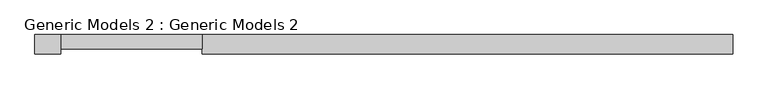
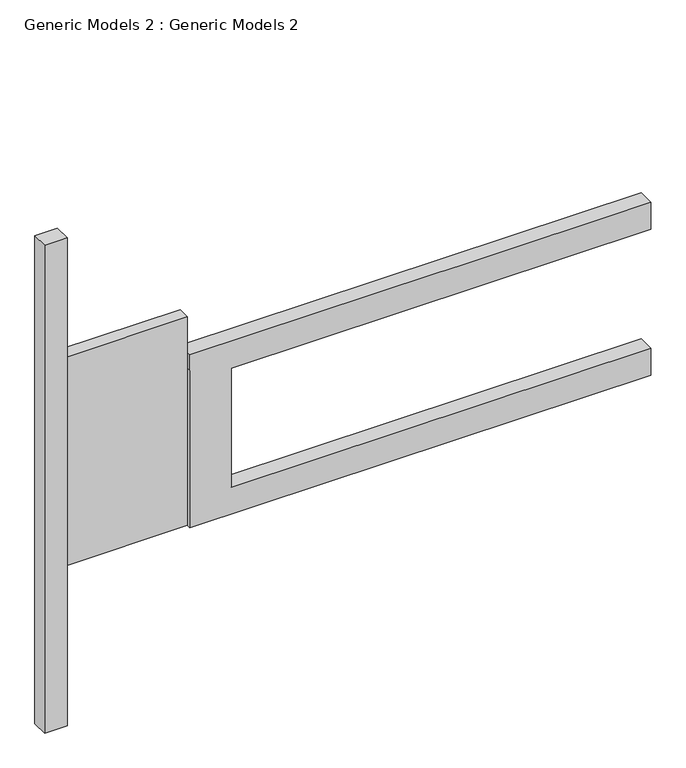
"""IFC4 building model written with IfcOpenShell, lengths in millimetres: proxy geometry, Generic Models 2 : Generic Models 2."""

from ifc_helpers import new_model, si_unit, frame, origin, place, context, project, spatial, polyline, outline, extrude, faceted_brep, source, transform, mapped, element, save


def generic_models_2_generic_models_2_3259aae0(model_context):
    return source(origin(), model_context, "Body", "SolidModel", [
        extrude(outline(polyline([(-14337.8476932, -15562.3742702), (-16587.1168969, -15562.3742702), (-16587.1168969, -15333.7742702), (-14337.8476932, -15333.7742702), (-14337.8476932, -15562.3742702)])), frame((0.0, 0.0, 3048.0), z_axis=(0.0, 0.0, 1.0), x_axis=(1.0, 0.0, 0.0)), (0.0, 0.0, 1.0), 4044.0651671),
        faceted_brep([(-16587.1168969, -15638.5742702, 9460.6359555), (-17001.1767684, -15638.5742702, 9460.6359555), (-17001.1767684, -15638.5742702, 9451.4798658), (-17001.1767684, -15638.5742702, 0.0), (-16587.1168969, -15638.5742702, 0.0), (-16587.1168969, -15638.5742702, 9451.4798658), (-16587.1168969, -15333.7742702, 9460.6359555), (-16587.1168969, -15333.7742702, 6400.8), (-16587.1168969, -15333.7742702, 0.0), (-17001.1767684, -15333.7742702, 0.0), (-17001.1767684, -15333.7742702, 6400.8), (-17001.1767684, -15333.7742702, 9460.6359555)], [[[0, 1, 2, 3, 4, 5]], [[6, 7, 8, 9, 10, 11]], [[1, 0, 6, 11]], [[3, 2, 1, 11, 10, 9]], [[4, 3, 9, 8]], [[0, 5, 4, 8, 7, 6]]]),
        faceted_brep([(-5875.9767684, -15638.5742702, 5877.1968868), (-5875.9767684, -15638.5742702, 6400.8), (-9360.4652876, -15638.5742702, 6400.8), (-9817.6652876, -15638.5742702, 6400.8), (-14332.4168407, -15638.5742702, 6400.8), (-14332.4168407, -15638.5742702, 6096.0), (-14337.8476932, -15638.5742702, 6096.0), (-14337.8476932, -15638.5742702, 3048.0), (-5875.9767684, -15638.5742702, 3048.0), (-5875.9767684, -15638.5742702, 3570.5755181), (-13572.1767684, -15638.5742702, 3570.5755181), (-13572.1767684, -15638.5742702, 5877.1968868), (-14332.4168407, -15333.7742702, 6400.8), (-5875.9767684, -15333.7742702, 6400.8), (-5875.9767684, -15333.7742702, 5877.1968868), (-13572.1767684, -15333.7742702, 5877.1968868), (-13572.1767684, -15333.7742702, 3570.5755181), (-5875.9767684, -15333.7742702, 3570.5755181), (-5875.9767684, -15333.7742702, 3048.0), (-14337.8476932, -15333.7742702, 3048.0), (-14337.8476932, -15333.7742702, 6096.0), (-14332.4168407, -15333.7742702, 6096.0)], [[[0, 1, 2, 3, 4, 5, 6, 7, 8, 9, 10, 11]], [[12, 13, 14, 15, 16, 17, 18, 19, 20, 21]], [[1, 0, 14, 13]], [[4, 3, 2, 1, 13, 12]], [[4, 12, 21, 5]], [[14, 0, 11, 15]], [[8, 7, 19, 18]], [[9, 8, 18, 17]], [[9, 17, 16, 10]], [[7, 6, 20, 19]], [[15, 11, 10, 16]], [[20, 6, 5, 21]]]),
    ])


if __name__ == "__main__":
    model = new_model("IFC4")
    model_context = context("Model", 3, world=origin())
    ifc_project = project(units=[si_unit("LENGTHUNIT", "METRE", prefix="MILLI")], contexts=[model_context])
    site = spatial("IfcSite", under=ifc_project)
    building = spatial("IfcBuilding", under=site)
    placement = place(None, origin())
    generic_models_2_generic_models_2_shape = generic_models_2_generic_models_2_3259aae0(model_context)
    element("IfcBuildingElementProxy", 1, Name="Generic Models 2 : Generic Models 2", ObjectType="Generic Models 2 : Generic Models 2", at=placement, inside=building, context=model_context, shape_type="MappedRepresentation", body=[
        mapped(generic_models_2_generic_models_2_shape, transform((0.0, 0.0, 0.0), x_axis=(1.0, 0.0, 0.0), y_axis=(0.0, 1.0, 0.0), z_axis=(0.0, 0.0, 1.0))),
    ])
    save(model, "model.ifc")
